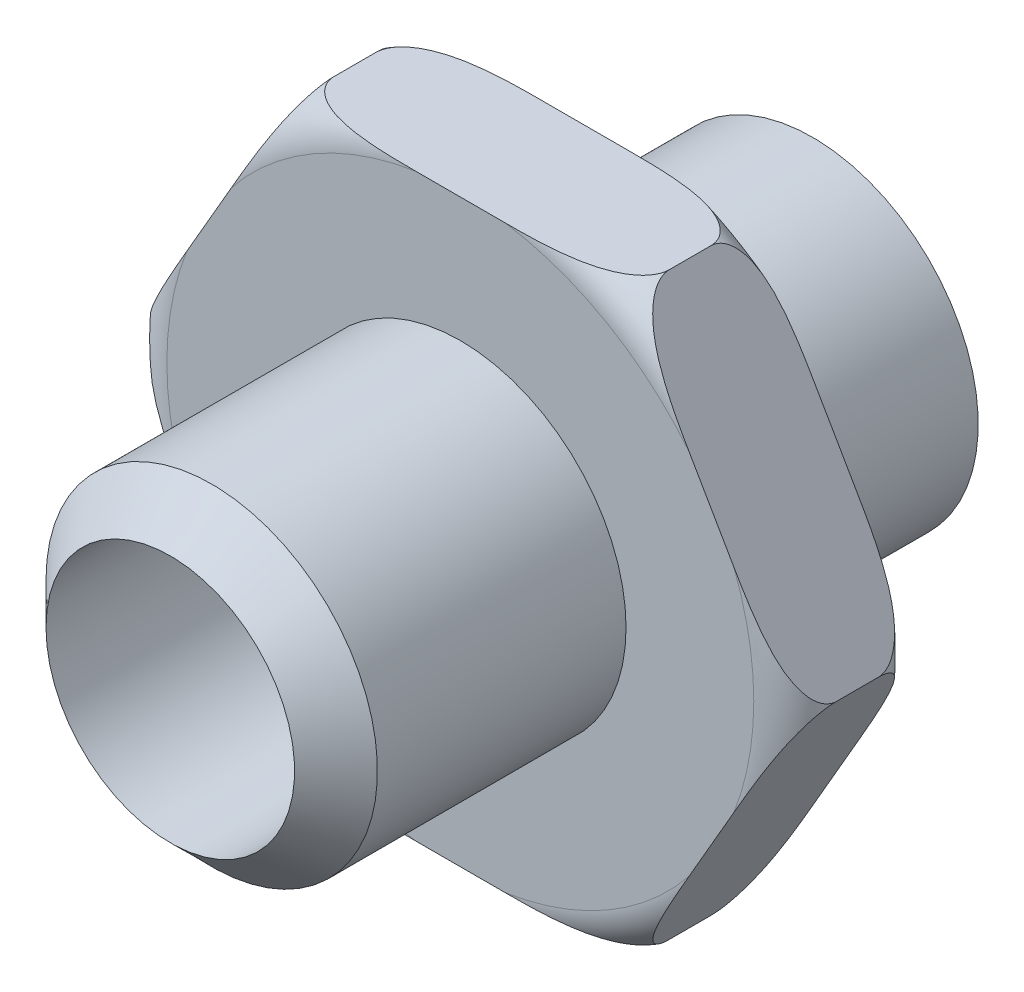
SolidWorks part; units mm, degrees
material "Plain Carbon Steel"
ref_plane "Front Plane" through (0, 0, 0) normal (0, 0, 1) x (1, 0, 0)
ref_plane "Top Plane" through (0, 0, 0) normal (0, 1, 0) x (1, 0, 0)
ref_plane "Right Plane" through (0, 0, 0) normal (1, 0, 0) x (0, 0, -1)
sketch "Hex Profile Sketch" plane through (0, 0, 0) normal (0, 0, 1) x (1, 0, 0)
  line L8 (8.0829, 14) -> (-8.0829, 14)
  line L9 (-8.0829, 14) -> (-16.1658, 0)
  line L10 (-16.1658, 0) -> (-8.0829, -14)
  line L11 (-8.0829, -14) -> (8.0829, -14)
  line L12 (8.0829, -14) -> (16.1658, 0)
  line L13 (16.1658, 0) -> (8.0829, 14)
  circle A0 centre (0, 0) radius 14 construction
  dimension "D1" = 28
extrude "Hex Body 28" add sketch "Hex Profile Sketch" against normal blind 6
sketch "Spigot Profile Sketch" plane through (0, 0, 0) normal (0, 1, 0) x (1, 0, 0)
  line L0 (0, 19.0302) -> (0, -16.2239) construction
  line L1 (0, 17) -> (-8, 17)
  line L2 (-8, 17) -> (-8, -7)
  line L3 (-8, -7) -> (-8, -15)
  line L5 (-8, -15) -> (0, -15)
  line L6 (0, 17) -> (0, -15)
  line L7 (8.0829, 6) -> (-8.0829, 6) construction
  dimension "D1" = 32
  dimension "D2" = 16
  dimension "D3" = 11
revolve "Threaded Spigots" add sketch "Spigot Profile Sketch" angle 360 about L0
cosmetic thread "Cosmetic Thread1" parameters "D1"=10, "D2"=13.797
chamfer "Spigot Chamfer 3x45" distance 3 angle 45 1 edges at (-8, 0, 15)
cosmetic thread "Cosmetic Thread2" parameters "D1"=10, "D2"=13.797
sketch "Bore Sketch Ø10" plane through (0, 0, -17) normal (0, 0, -1) x (-1, 0, 0)
  circle A0 centre (0, 0) radius 6
  dimension "D1" = 12
extrude "Through Bore Ø10" cut sketch "Bore Sketch Ø10" against normal up to next
sketch "Thread Groove Profile Sketch" plane through (0, 0, 0) normal (0, 1, 0) x (1, 0, 0)
  line L0 (-16.1658, 6) -> (-16.1658, 0) construction
  line L1 (-8.0829, 6) -> (-16.1658, 6) construction
  line L2 (-14.1658, 6) -> (-16.1658, 6)
  line L3 (-16.1658, 6) -> (-16.1658, 4)
  line L4 (0, 0) -> (0, 20.0495) construction
  line L5 (-18.6573, 3) -> (-10.4323, 3) construction
  line L6 (-16.1658, 0) -> (-16.1658, 2)
  line L7 (-14.1658, 0) -> (-16.1658, 0)
  arc A0 (-16.1658, 4) -> (-14.1658, 6) centre (-14.1658, 4) cw
  arc A1 (-16.1658, 2) -> (-14.1658, 0) centre (-14.1658, 2) ccw
  dimension "D1" = 2
  dimension "D2" = 3
revolve "Thread Grooves" cut sketch "Thread Groove Profile Sketch" angle 360 about L4
